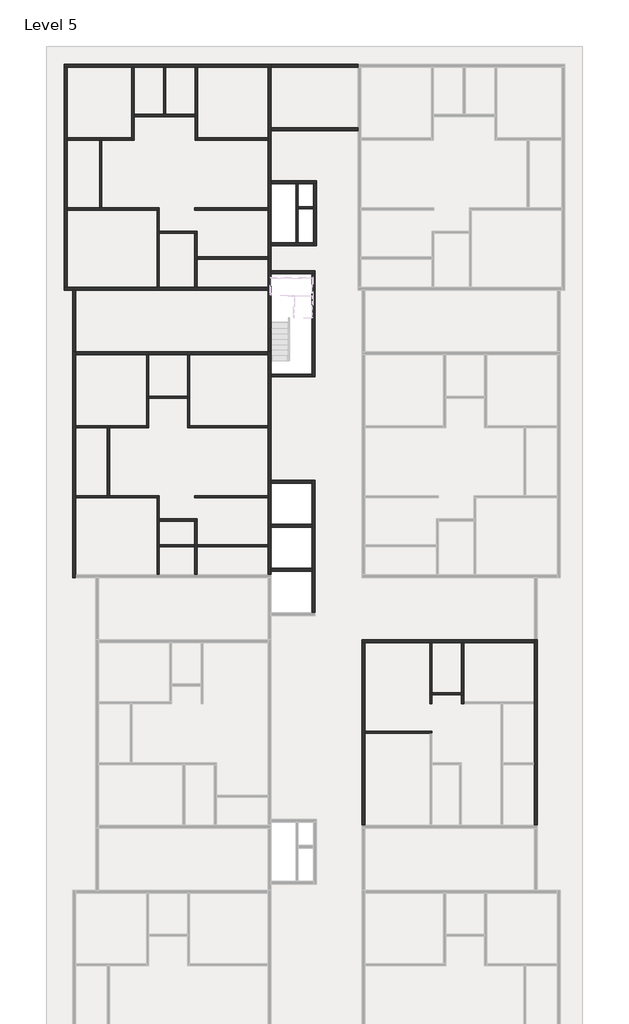
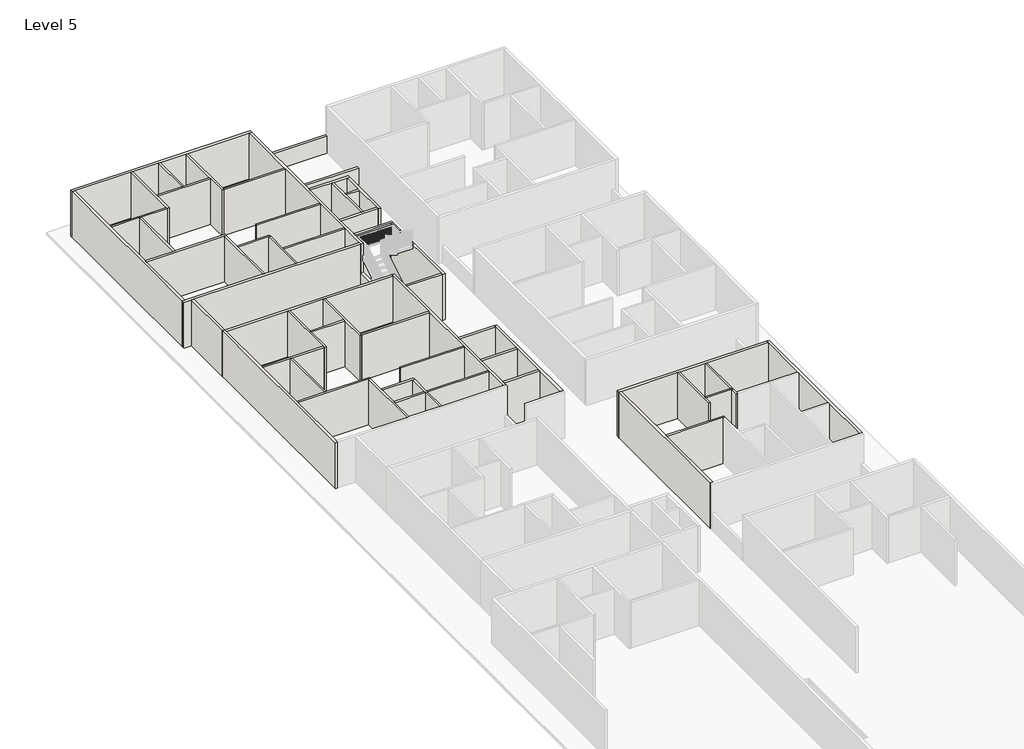
# One storey, part 3 of 8: 57 walls.
"""IFC4 building model written with IfcOpenShell, lengths in millimetres."""

from ifc_helpers import new_model, si_unit, frame, origin, place, context, project, spatial, polyline, outline, extrude, faceted_brep, element, save

model = new_model("IFC4")

# Units and contexts
model_context = context("Model", 3, world=origin())
ifc_project = project(units=[si_unit("LENGTHUNIT", "METRE", prefix="MILLI")], contexts=[model_context])

# Site, building, storey
site = spatial("IfcSite", under=ifc_project)
building = spatial("IfcBuilding", under=site)
storey = spatial("IfcBuildingStorey", under=building, Name="Level 5", Elevation=37426.6172466)

# Walls
placement = place(None, origin())
element("IfcWall", 1, ObjectType="4.5\"", at=placement, inside=storey, context=model_context, shape_type="Brep", body=[
    faceted_brep([(-10818.3415084, 35031.1216096, 37426.6172466), (-10818.3415084, 31373.5216096, 37426.6172466), (-10818.3415084, 31259.2216096, 37426.6172466), (-10818.3415084, 31259.2216096, 40474.6172466), (-10818.3415084, 31373.5216096, 40474.6172466), (-10818.3415084, 35031.1216096, 40474.6172466), (-10704.0415084, 35031.1216096, 37426.6172466), (-10704.0415084, 35031.1216096, 40474.6172466), (-10704.0415084, 32592.7216096, 40474.6172466), (-10704.0415084, 32478.4216096, 40474.6172466), (-10704.0415084, 31259.2216096, 40474.6172466), (-10704.0415084, 31259.2216096, 37426.6172466), (-10704.0415084, 32478.4216096, 37426.6172466), (-10704.0415084, 32592.7216096, 37426.6172466)], [[[0, 1, 2, 3, 4, 5]], [[6, 7, 8, 9, 10, 11, 12, 13]], [[2, 1, 0, 6, 13, 12, 11]], [[0, 5, 7, 6]], [[3, 2, 11, 10]], [[5, 4, 3, 10, 9, 8, 7]]]),
])
element("IfcWall", 2, ObjectType="4.5\"", at=placement, inside=storey, context=model_context, shape_type="Brep", body=[
    faceted_brep([(-10818.3415084, 31373.5216096, 37426.6172466), (-14171.1415084, 31373.5216096, 37426.6172466), (-14171.1415084, 31373.5216096, 40474.6172466), (-10818.3415084, 31373.5216096, 40474.6172466), (-10818.3415084, 31259.2216096, 37426.6172466), (-10818.3415084, 31259.2216096, 40474.6172466), (-12380.4415084, 31259.2216096, 40474.6172466), (-12494.7415084, 31259.2216096, 40474.6172466), (-14171.1415084, 31259.2216096, 40474.6172466), (-14171.1415084, 31259.2216096, 37426.6172466), (-12494.7415084, 31259.2216096, 37426.6172466), (-12380.4415084, 31259.2216096, 37426.6172466)], [[[0, 1, 2, 3]], [[4, 5, 6, 7, 8, 9, 10, 11]], [[1, 0, 4, 11, 10, 9]], [[0, 3, 5, 4]], [[2, 1, 9, 8]], [[3, 2, 8, 7, 6, 5]]]),
])
element("IfcWall", 3, ObjectType="4.5\"", at=placement, inside=storey, context=model_context, shape_type="SweptSolid", body=[
    extrude(outline(polyline([(-12494.7415084, 27754.0216096), (-12494.7415084, 31259.2216096), (-12380.4415084, 31259.2216096), (-12380.4415084, 27754.0216096), (-12494.7415084, 27754.0216096)])), frame((0.0, 0.0, 37426.6172466), z_axis=(0.0, 0.0, 1.0), x_axis=(1.0, 0.0, 0.0)), (0.0, 0.0, 1.0), 3048.0),
])
element("IfcWall", 4, ObjectType="4.5\"", at=placement, inside=storey, context=model_context, shape_type="Brep", body=[
    faceted_brep([(-14171.1415084, 27639.7216096, 37426.6172466), (-9510.2415084, 27639.7216096, 37426.6172466), (-9395.9415084, 27639.7216096, 37426.6172466), (-9395.9415084, 27639.7216096, 40474.6172466), (-9510.2415084, 27639.7216096, 40474.6172466), (-14171.1415084, 27639.7216096, 40474.6172466), (-14171.1415084, 27754.0216096, 37426.6172466), (-14171.1415084, 27754.0216096, 40474.6172466), (-12494.7415084, 27754.0216096, 40474.6172466), (-12380.4415084, 27754.0216096, 40474.6172466), (-9395.9415084, 27754.0216096, 40474.6172466), (-9395.9415084, 27754.0216096, 37426.6172466), (-12380.4415084, 27754.0216096, 37426.6172466), (-12494.7415084, 27754.0216096, 37426.6172466)], [[[0, 1, 2, 3, 4, 5]], [[6, 7, 8, 9, 10, 11, 12, 13]], [[2, 1, 0, 6, 13, 12, 11]], [[0, 5, 7, 6]], [[3, 2, 11, 10]], [[5, 4, 3, 10, 9, 8, 7]]]),
])
element("IfcWall", 5, ObjectType="4.5\"", at=placement, inside=storey, context=model_context, shape_type="Brep", body=[
    faceted_brep([(-9510.2415084, 27639.7216096, 37426.6172466), (-9510.2415084, 23651.9216096, 37426.6172466), (-9510.2415084, 23651.9216096, 40474.6172466), (-9510.2415084, 27639.7216096, 40474.6172466), (-9395.9415084, 27639.7216096, 37426.6172466), (-9395.9415084, 27639.7216096, 40474.6172466), (-9395.9415084, 26547.5216096, 40474.6172466), (-9395.9415084, 26433.2216096, 40474.6172466), (-9395.9415084, 23651.9216096, 40474.6172466), (-9395.9415084, 23651.9216096, 37426.6172466), (-9395.9415084, 26433.2216096, 37426.6172466), (-9395.9415084, 26547.5216096, 37426.6172466)], [[[0, 1, 2, 3]], [[4, 5, 6, 7, 8, 9, 10, 11]], [[1, 0, 4, 11, 10, 9]], [[0, 3, 5, 4]], [[2, 1, 9, 8]], [[3, 2, 8, 7, 6, 5]]]),
])
element("IfcWall", 6, ObjectType="4.5\"", at=placement, inside=storey, context=model_context, shape_type="Brep", body=[
    faceted_brep([(-9395.9415084, 26433.2216096, 37426.6172466), (-7567.1415084, 26433.2216096, 37426.6172466), (-7452.8415084, 26433.2216096, 37426.6172466), (-7452.8415084, 26433.2216096, 40474.6172466), (-7567.1415084, 26433.2216096, 40474.6172466), (-9395.9415084, 26433.2216096, 40474.6172466), (-9395.9415084, 26547.5216096, 37426.6172466), (-9395.9415084, 26547.5216096, 40474.6172466), (-7452.8415084, 26547.5216096, 40474.6172466), (-7452.8415084, 26547.5216096, 37426.6172466)], [[[0, 1, 2, 3, 4, 5]], [[6, 7, 8, 9]], [[2, 1, 0, 6, 9]], [[0, 5, 7, 6]], [[3, 2, 9, 8]], [[5, 4, 3, 8, 7]]]),
])
element("IfcWall", 7, ObjectType="4.5\"", at=placement, inside=storey, context=model_context, shape_type="Brep", body=[
    faceted_brep([(-7567.1415084, 26433.2216096, 37426.6172466), (-7567.1415084, 23651.9216096, 37426.6172466), (-7567.1415084, 23651.9216096, 40474.6172466), (-7567.1415084, 26433.2216096, 40474.6172466), (-7452.8415084, 26433.2216096, 37426.6172466), (-7452.8415084, 26433.2216096, 40474.6172466), (-7452.8415084, 25214.0216096, 40474.6172466), (-7452.8415084, 25099.7216096, 40474.6172466), (-7452.8415084, 23651.9216096, 40474.6172466), (-7452.8415084, 23651.9216096, 37426.6172466), (-7452.8415084, 25099.7216096, 37426.6172466), (-7452.8415084, 25214.0216096, 37426.6172466)], [[[0, 1, 2, 3]], [[4, 5, 6, 7, 8, 9, 10, 11]], [[1, 0, 4, 11, 10, 9]], [[0, 3, 5, 4]], [[2, 1, 9, 8]], [[3, 2, 8, 7, 6, 5]]]),
])
element("IfcWall", 8, ObjectType="4.5\"", at=placement, inside=storey, context=model_context, shape_type="SweptSolid", body=[
    extrude(outline(polyline([(-7452.8415084, 25214.0216096), (-3769.8415084, 25214.0216096), (-3769.8415084, 25099.7216096), (-7452.8415084, 25099.7216096), (-7452.8415084, 25214.0216096)])), frame((0.0, 0.0, 37426.6172466), z_axis=(0.0, 0.0, 1.0), x_axis=(1.0, 0.0, 0.0)), (0.0, 0.0, 1.0), 3048.0),
])
element("IfcWall", 9, ObjectType="4.5\"", at=placement, inside=storey, context=model_context, shape_type="SweptSolid", body=[
    extrude(outline(polyline([(-3769.8415084, 27639.7216096), (-7567.1415084, 27639.7216096), (-7567.1415084, 27754.0216096), (-3769.8415084, 27754.0216096), (-3769.8415084, 27639.7216096)])), frame((0.0, 0.0, 37426.6172466), z_axis=(0.0, 0.0, 1.0), x_axis=(1.0, 0.0, 0.0)), (0.0, 0.0, 1.0), 3048.0),
])
element("IfcWall", 10, ObjectType="4.5\"", at=placement, inside=storey, context=model_context, shape_type="Brep", body=[
    faceted_brep([(-10704.0415084, 32478.4216096, 37426.6172466), (-7541.7415084, 32478.4216096, 37426.6172466), (-7541.7415084, 32478.4216096, 40474.6172466), (-10704.0415084, 32478.4216096, 40474.6172466), (-10704.0415084, 32592.7216096, 37426.6172466), (-10704.0415084, 32592.7216096, 40474.6172466), (-9180.0415084, 32592.7216096, 40474.6172466), (-9065.7415084, 32592.7216096, 40474.6172466), (-7541.7415084, 32592.7216096, 40474.6172466), (-7541.7415084, 32592.7216096, 37426.6172466), (-9065.7415084, 32592.7216096, 37426.6172466), (-9180.0415084, 32592.7216096, 37426.6172466)], [[[0, 1, 2, 3]], [[4, 5, 6, 7, 8, 9, 10, 11]], [[1, 0, 4, 11, 10, 9]], [[0, 3, 5, 4]], [[2, 1, 9, 8]], [[3, 2, 8, 7, 6, 5]]]),
])
element("IfcWall", 11, ObjectType="4.5\"", at=placement, inside=storey, context=model_context, shape_type="SweptSolid", body=[
    extrude(outline(polyline([(-9180.0415084, 32592.7216096), (-9180.0415084, 35031.1216096), (-9065.7415084, 35031.1216096), (-9065.7415084, 32592.7216096), (-9180.0415084, 32592.7216096)])), frame((0.0, 0.0, 37426.6172466), z_axis=(0.0, 0.0, 1.0), x_axis=(1.0, 0.0, 0.0)), (0.0, 0.0, 1.0), 3048.0),
])
element("IfcWall", 12, ObjectType="4.5\"", at=placement, inside=storey, context=model_context, shape_type="Brep", body=[
    faceted_brep([(-7541.7415084, 35031.1216096, 37426.6172466), (-7541.7415084, 32592.7216096, 37426.6172466), (-7541.7415084, 32478.4216096, 37426.6172466), (-7541.7415084, 31259.2216096, 37426.6172466), (-7541.7415084, 31259.2216096, 40474.6172466), (-7541.7415084, 32478.4216096, 40474.6172466), (-7541.7415084, 32592.7216096, 40474.6172466), (-7541.7415084, 35031.1216096, 40474.6172466), (-7427.4415084, 35031.1216096, 37426.6172466), (-7427.4415084, 35031.1216096, 40474.6172466), (-7427.4415084, 31373.5216096, 40474.6172466), (-7427.4415084, 31259.2216096, 40474.6172466), (-7427.4415084, 31259.2216096, 37426.6172466), (-7427.4415084, 31373.5216096, 37426.6172466)], [[[0, 1, 2, 3, 4, 5, 6, 7]], [[8, 9, 10, 11, 12, 13]], [[3, 2, 1, 0, 8, 13, 12]], [[0, 7, 9, 8]], [[4, 3, 12, 11]], [[7, 6, 5, 4, 11, 10, 9]]]),
])
element("IfcWall", 13, ObjectType="4.5\"", at=placement, inside=storey, context=model_context, shape_type="SweptSolid", body=[
    extrude(outline(polyline([(-3769.8415084, 31259.2216096), (-7427.4415084, 31259.2216096), (-7427.4415084, 31373.5216096), (-3769.8415084, 31373.5216096), (-3769.8415084, 31259.2216096)])), frame((0.0, 0.0, 37426.6172466), z_axis=(0.0, 0.0, 1.0), x_axis=(1.0, 0.0, 0.0)), (0.0, 0.0, 1.0), 3048.0),
])
element("IfcWall", 14, ObjectType="4.5\"", at=placement, inside=storey, context=model_context, shape_type="Brep", body=[
    faceted_brep([(-10061.4044854, 20146.7216096, 37426.6172466), (-10061.4044854, 16489.1216096, 37426.6172466), (-10061.4044854, 16374.8216096, 37426.6172466), (-10061.4044854, 16374.8216096, 40474.6172466), (-10061.4044854, 16489.1216096, 40474.6172466), (-10061.4044854, 20146.7216096, 40474.6172466), (-9947.1044854, 20146.7216096, 37426.6172466), (-9947.1044854, 20146.7216096, 40474.6172466), (-9947.1044854, 18013.1216096, 40474.6172466), (-9947.1044854, 17898.8216096, 40474.6172466), (-9947.1044854, 16374.8216096, 40474.6172466), (-9947.1044854, 16374.8216096, 37426.6172466), (-9947.1044854, 17898.8216096, 37426.6172466), (-9947.1044854, 18013.1216096, 37426.6172466)], [[[0, 1, 2, 3, 4, 5]], [[6, 7, 8, 9, 10, 11, 12, 13]], [[2, 1, 0, 6, 13, 12, 11]], [[0, 5, 7, 6]], [[3, 2, 11, 10]], [[5, 4, 3, 10, 9, 8, 7]]]),
])
element("IfcWall", 15, ObjectType="4.5\"", at=placement, inside=storey, context=model_context, shape_type="Brep", body=[
    faceted_brep([(-10061.4044854, 16489.1216096, 37426.6172466), (-13719.0044854, 16489.1216096, 37426.6172466), (-13719.0044854, 16489.1216096, 40474.6172466), (-10061.4044854, 16489.1216096, 40474.6172466), (-10061.4044854, 16374.8216096, 37426.6172466), (-10061.4044854, 16374.8216096, 40474.6172466), (-11980.3915084, 16374.8216096, 40474.6172466), (-12094.6915084, 16374.8216096, 40474.6172466), (-13719.0044854, 16374.8216096, 40474.6172466), (-13719.0044854, 16374.8216096, 37426.6172466), (-12094.6915084, 16374.8216096, 37426.6172466), (-11980.3915084, 16374.8216096, 37426.6172466)], [[[0, 1, 2, 3]], [[4, 5, 6, 7, 8, 9, 10, 11]], [[1, 0, 4, 11, 10, 9]], [[0, 3, 5, 4]], [[2, 1, 9, 8]], [[3, 2, 8, 7, 6, 5]]]),
])
element("IfcWall", 16, ObjectType="4.5\"", at=placement, inside=storey, context=model_context, shape_type="SweptSolid", body=[
    extrude(outline(polyline([(-7940.5044854, 17898.8216096), (-9947.1044854, 17898.8216096), (-9947.1044854, 18013.1216096), (-7940.5044854, 18013.1216096), (-7940.5044854, 17898.8216096)])), frame((0.0, 0.0, 37426.6172466), z_axis=(0.0, 0.0, 1.0), x_axis=(1.0, 0.0, 0.0)), (0.0, 0.0, 1.0), 3048.0),
])
element("IfcWall", 17, ObjectType="4.5\"", at=placement, inside=storey, context=model_context, shape_type="Brep", body=[
    faceted_brep([(-7940.5044854, 20146.7216096, 37426.6172466), (-7940.5044854, 18013.1216096, 37426.6172466), (-7940.5044854, 17898.8216096, 37426.6172466), (-7940.5044854, 16374.8216096, 37426.6172466), (-7940.5044854, 16374.8216096, 40474.6172466), (-7940.5044854, 17898.8216096, 40474.6172466), (-7940.5044854, 18013.1216096, 40474.6172466), (-7940.5044854, 20146.7216096, 40474.6172466), (-7826.2044854, 20146.7216096, 37426.6172466), (-7826.2044854, 20146.7216096, 40474.6172466), (-7826.2044854, 16489.1216096, 40474.6172466), (-7826.2044854, 16374.8216096, 40474.6172466), (-7826.2044854, 16374.8216096, 37426.6172466), (-7826.2044854, 16489.1216096, 37426.6172466)], [[[0, 1, 2, 3, 4, 5, 6, 7]], [[8, 9, 10, 11, 12, 13]], [[3, 2, 1, 0, 8, 13, 12]], [[0, 7, 9, 8]], [[4, 3, 12, 11]], [[7, 6, 5, 4, 11, 10, 9]]]),
])
element("IfcWall", 18, ObjectType="4.5\"", at=placement, inside=storey, context=model_context, shape_type="SweptSolid", body=[
    extrude(outline(polyline([(-3769.8415084, 16374.8216096), (-7826.2044854, 16374.8216096), (-7826.2044854, 16489.1216096), (-3769.8415084, 16489.1216096), (-3769.8415084, 16374.8216096)])), frame((0.0, 0.0, 37426.6172466), z_axis=(0.0, 0.0, 1.0), x_axis=(1.0, 0.0, 0.0)), (0.0, 0.0, 1.0), 3048.0),
])
element("IfcWall", 19, ObjectType="4.5\"", at=placement, inside=storey, context=model_context, shape_type="SweptSolid", body=[
    extrude(outline(polyline([(-12094.6915084, 12869.6216096), (-12094.6915084, 16374.8216096), (-11980.3915084, 16374.8216096), (-11980.3915084, 12869.6216096), (-12094.6915084, 12869.6216096)])), frame((0.0, 0.0, 37426.6172466), z_axis=(0.0, 0.0, 1.0), x_axis=(1.0, 0.0, 0.0)), (0.0, 0.0, 1.0), 3048.0),
])
element("IfcWall", 20, ObjectType="4.5\"", at=placement, inside=storey, context=model_context, shape_type="Brep", body=[
    faceted_brep([(-13719.0044854, 12755.3216096, 37426.6172466), (-9510.2415084, 12755.3216096, 37426.6172466), (-9395.9415084, 12755.3216096, 37426.6172466), (-9395.9415084, 12755.3216096, 40474.6172466), (-9510.2415084, 12755.3216096, 40474.6172466), (-13719.0044854, 12755.3216096, 40474.6172466), (-13719.0044854, 12869.6216096, 37426.6172466), (-13719.0044854, 12869.6216096, 40474.6172466), (-12094.6915084, 12869.6216096, 40474.6172466), (-11980.3915084, 12869.6216096, 40474.6172466), (-9395.9415084, 12869.6216096, 40474.6172466), (-9395.9415084, 12869.6216096, 37426.6172466), (-11980.3915084, 12869.6216096, 37426.6172466), (-12094.6915084, 12869.6216096, 37426.6172466)], [[[0, 1, 2, 3, 4, 5]], [[6, 7, 8, 9, 10, 11, 12, 13]], [[2, 1, 0, 6, 13, 12, 11]], [[0, 5, 7, 6]], [[3, 2, 11, 10]], [[5, 4, 3, 10, 9, 8, 7]]]),
])
element("IfcWall", 21, ObjectType="4.5\"", at=placement, inside=storey, context=model_context, shape_type="Brep", body=[
    faceted_brep([(-9510.2415084, 12755.3216096, 37426.6172466), (-9510.2415084, 8767.5216096, 37426.6172466), (-9510.2415084, 8767.5216096, 40474.6172466), (-9510.2415084, 12755.3216096, 40474.6172466), (-9395.9415084, 12755.3216096, 37426.6172466), (-9395.9415084, 12755.3216096, 40474.6172466), (-9395.9415084, 11663.1216096, 40474.6172466), (-9395.9415084, 11548.8216096, 40474.6172466), (-9395.9415084, 10329.6216096, 40474.6172466), (-9395.9415084, 10215.3216096, 40474.6172466), (-9395.9415084, 8767.5216096, 40474.6172466), (-9395.9415084, 8767.5216096, 37426.6172466), (-9395.9415084, 10215.3216096, 37426.6172466), (-9395.9415084, 10329.6216096, 37426.6172466), (-9395.9415084, 11548.8216096, 37426.6172466), (-9395.9415084, 11663.1216096, 37426.6172466)], [[[0, 1, 2, 3]], [[4, 5, 6, 7, 8, 9, 10, 11, 12, 13, 14, 15]], [[1, 0, 4, 15, 14, 13, 12, 11]], [[0, 3, 5, 4]], [[2, 1, 11, 10]], [[3, 2, 10, 9, 8, 7, 6, 5]]]),
])
element("IfcWall", 22, ObjectType="4.5\"", at=placement, inside=storey, context=model_context, shape_type="SweptSolid", body=[
    extrude(outline(polyline([(-7567.1415084, 10215.3216096), (-9395.9415084, 10215.3216096), (-9395.9415084, 10329.6216096), (-7567.1415084, 10329.6216096), (-7567.1415084, 10215.3216096)])), frame((0.0, 0.0, 37426.6172466), z_axis=(0.0, 0.0, 1.0), x_axis=(1.0, 0.0, 0.0)), (0.0, 0.0, 1.0), 3048.0),
])
element("IfcWall", 23, ObjectType="4.5\"", at=placement, inside=storey, context=model_context, shape_type="Brep", body=[
    faceted_brep([(-9395.9415084, 11548.8216096, 37426.6172466), (-7567.1415084, 11548.8216096, 37426.6172466), (-7452.8415084, 11548.8216096, 37426.6172466), (-7452.8415084, 11548.8216096, 40474.6172466), (-7567.1415084, 11548.8216096, 40474.6172466), (-9395.9415084, 11548.8216096, 40474.6172466), (-9395.9415084, 11663.1216096, 37426.6172466), (-9395.9415084, 11663.1216096, 40474.6172466), (-7452.8415084, 11663.1216096, 40474.6172466), (-7452.8415084, 11663.1216096, 37426.6172466)], [[[0, 1, 2, 3, 4, 5]], [[6, 7, 8, 9]], [[2, 1, 0, 6, 9]], [[0, 5, 7, 6]], [[3, 2, 9, 8]], [[5, 4, 3, 8, 7]]]),
])
element("IfcWall", 24, ObjectType="4.5\"", at=placement, inside=storey, context=model_context, shape_type="Brep", body=[
    faceted_brep([(-7567.1415084, 11548.8216096, 37426.6172466), (-7567.1415084, 10329.6216096, 37426.6172466), (-7567.1415084, 10215.3216096, 37426.6172466), (-7567.1415084, 8767.5216096, 37426.6172466), (-7567.1415084, 8767.5216096, 40474.6172466), (-7567.1415084, 10215.3216096, 40474.6172466), (-7567.1415084, 10329.6216096, 40474.6172466), (-7567.1415084, 11548.8216096, 40474.6172466), (-7452.8415084, 11548.8216096, 37426.6172466), (-7452.8415084, 11548.8216096, 40474.6172466), (-7452.8415084, 10329.6216096, 40474.6172466), (-7452.8415084, 10215.3216096, 40474.6172466), (-7452.8415084, 8767.5216096, 40474.6172466), (-7452.8415084, 8767.5216096, 37426.6172466), (-7452.8415084, 10215.3216096, 37426.6172466), (-7452.8415084, 10329.6216096, 37426.6172466)], [[[0, 1, 2, 3, 4, 5, 6, 7]], [[8, 9, 10, 11, 12, 13, 14, 15]], [[3, 2, 1, 0, 8, 15, 14, 13]], [[0, 7, 9, 8]], [[4, 3, 13, 12]], [[7, 6, 5, 4, 12, 11, 10, 9]]]),
])
element("IfcWall", 25, ObjectType="4.5\"", at=placement, inside=storey, context=model_context, shape_type="SweptSolid", body=[
    extrude(outline(polyline([(-3769.8415084, 10215.3216096), (-7452.8415084, 10215.3216096), (-7452.8415084, 10329.6216096), (-3769.8415084, 10329.6216096), (-3769.8415084, 10215.3216096)])), frame((0.0, 0.0, 37426.6172466), z_axis=(0.0, 0.0, 1.0), x_axis=(1.0, 0.0, 0.0)), (0.0, 0.0, 1.0), 3048.0),
])
element("IfcWall", 26, ObjectType="4.5\"", at=placement, inside=storey, context=model_context, shape_type="SweptSolid", body=[
    extrude(outline(polyline([(-3769.8415084, 12755.3216096), (-7567.1415084, 12755.3216096), (-7567.1415084, 12869.6216096), (-3769.8415084, 12869.6216096), (-3769.8415084, 12755.3216096)])), frame((0.0, 0.0, 37426.6172466), z_axis=(0.0, 0.0, 1.0), x_axis=(1.0, 0.0, 0.0)), (0.0, 0.0, 1.0), 3048.0),
])
element("IfcWall", 27, ObjectType="4.5\"", at=placement, inside=storey, context=model_context, shape_type="Brep", body=[
    faceted_brep([(1259.3584916, 572.7745083, 37426.6172466), (4610.8714687, 572.7745083, 37426.6172466), (4725.1714687, 572.7745083, 37426.6172466), (4725.1714687, 572.7745083, 40474.6172466), (4610.8714687, 572.7745083, 40474.6172466), (1259.3584916, 572.7745083, 40474.6172466), (1259.3584916, 687.0745083, 37426.6172466), (1259.3584916, 687.0745083, 40474.6172466), (4725.1714687, 687.0745083, 40474.6172466), (4725.1714687, 687.0745083, 37426.6172466)], [[[0, 1, 2, 3, 4, 5]], [[6, 7, 8, 9]], [[2, 1, 0, 6, 9]], [[0, 5, 7, 6]], [[3, 2, 9, 8]], [[5, 4, 3, 8, 7]]]),
])
element("IfcWall", 28, ObjectType="4.5\"", at=placement, inside=storey, context=model_context, shape_type="Brep", body=[
    faceted_brep([(4610.8714687, 5262.3216096, 37426.6172466), (4610.8714687, 2100.0216096, 37426.6172466), (4610.8714687, 2100.0216096, 40474.6172466), (4610.8714687, 5262.3216096, 40474.6172466), (4725.1714687, 5262.3216096, 37426.6172466), (4725.1714687, 5262.3216096, 40474.6172466), (4725.1714687, 2671.5216096, 40474.6172466), (4725.1714687, 2557.2216096, 40474.6172466), (4725.1714687, 2100.0216096, 40474.6172466), (4725.1714687, 2100.0216096, 37426.6172466), (4725.1714687, 2557.2216096, 37426.6172466), (4725.1714687, 2671.5216096, 37426.6172466)], [[[0, 1, 2, 3]], [[4, 5, 6, 7, 8, 9, 10, 11]], [[1, 0, 4, 11, 10, 9]], [[2, 1, 9, 8]], [[0, 3, 5, 4]], [[3, 2, 8, 7, 6, 5]]]),
])
element("IfcWall", 29, ObjectType="4.5\"", at=placement, inside=storey, context=model_context, shape_type="Brep", body=[
    faceted_brep([(4725.1714687, 2557.2216096, 37426.6172466), (6249.1714687, 2557.2216096, 37426.6172466), (6363.4714687, 2557.2216096, 37426.6172466), (6363.4714687, 2557.2216096, 40474.6172466), (6249.1714687, 2557.2216096, 40474.6172466), (4725.1714687, 2557.2216096, 40474.6172466), (4725.1714687, 2671.5216096, 37426.6172466), (4725.1714687, 2671.5216096, 40474.6172466), (6249.1714687, 2671.5216096, 40474.6172466), (6363.4714687, 2671.5216096, 40474.6172466), (6363.4714687, 2671.5216096, 37426.6172466), (6249.1714687, 2671.5216096, 37426.6172466)], [[[0, 1, 2, 3, 4, 5]], [[6, 7, 8, 9, 10, 11]], [[2, 1, 0, 6, 11, 10]], [[0, 5, 7, 6]], [[3, 2, 10, 9]], [[5, 4, 3, 9, 8, 7]]]),
])
element("IfcWall", 30, ObjectType="4.5\"", at=placement, inside=storey, context=model_context, shape_type="SweptSolid", body=[
    extrude(outline(polyline([(6363.4714687, 5262.3216096), (6363.4714687, 2671.5216096), (6249.1714687, 2671.5216096), (6249.1714687, 5262.3216096), (6363.4714687, 5262.3216096)])), frame((0.0, 0.0, 37426.6172466), z_axis=(0.0, 0.0, 1.0), x_axis=(1.0, 0.0, 0.0)), (0.0, 0.0, 1.0), 3048.0),
])
element("IfcWall", 31, ObjectType="4.5\"", at=placement, inside=storey, context=model_context, shape_type="Brep", body=[
    faceted_brep([(6249.1714687, 2557.2216096, 37426.6172466), (6249.1714687, 2100.0216096, 37426.6172466), (6249.1714687, 2100.0216096, 40474.6172466), (6249.1714687, 2557.2216096, 40474.6172466), (6363.4714687, 2557.2216096, 37426.6172466), (6363.4714687, 2557.2216096, 40474.6172466), (6363.4714687, 2214.3216096, 40474.6172466), (6363.4714687, 2100.0216096, 40474.6172466), (6363.4714687, 2100.0216096, 37426.6172466), (6363.4714687, 2214.3216096, 37426.6172466)], [[[0, 1, 2, 3]], [[4, 5, 6, 7, 8, 9]], [[1, 0, 4, 9, 8]], [[0, 3, 5, 4]], [[2, 1, 8, 7]], [[3, 2, 7, 6, 5]]]),
])
element("IfcWall", 32, ObjectType="4.5\"", at=placement, inside=storey, context=model_context, shape_type="Brep", body=[
    faceted_brep([(-2321.9738684, 29000.0900967, 37426.6172466), (-2321.9738684, 25952.0900967, 37426.6172466), (-2321.9738684, 25952.0900967, 40474.6172466), (-2321.9738684, 29000.0900967, 40474.6172466), (-2207.6738684, 29000.0900967, 37426.6172466), (-2207.6738684, 29000.0900967, 40474.6172466), (-2207.6738684, 27820.8172885, 40474.6172466), (-2207.6738684, 27706.5172885, 40474.6172466), (-2207.6738684, 25952.0900967, 40474.6172466), (-2207.6738684, 25952.0900967, 37426.6172466), (-2207.6738684, 27706.5172885, 37426.6172466), (-2207.6738684, 27820.8172885, 37426.6172466)], [[[0, 1, 2, 3]], [[4, 5, 6, 7, 8, 9, 10, 11]], [[1, 0, 4, 11, 10, 9]], [[3, 2, 8, 7, 6, 5]], [[0, 3, 5, 4]], [[2, 1, 9, 8]]]),
])
element("IfcWall", 33, ObjectType="4.5\"", at=placement, inside=storey, context=model_context, shape_type="SweptSolid", body=[
    extrude(outline(polyline([(-2207.6738684, 27820.8172885), (-1407.6415084, 27820.8172885), (-1407.6415084, 27706.5172885), (-2207.6738684, 27706.5172885), (-2207.6738684, 27820.8172885)])), frame((0.0, 0.0, 37426.6172466), z_axis=(0.0, 0.0, 1.0), x_axis=(1.0, 0.0, 0.0)), (0.0, 0.0, 1.0), 3048.0),
])
element("IfcWall", 34, ObjectType="6\"", at=placement, inside=storey, context=model_context, shape_type="Brep", body=[
    faceted_brep([(-14323.5415084, 35031.1216096, 37426.6172466), (-14171.1415084, 35031.1216096, 37426.6172466), (-10818.3415084, 35031.1216096, 37426.6172466), (-10704.0415084, 35031.1216096, 37426.6172466), (-9180.0415084, 35031.1216096, 37426.6172466), (-9065.7415084, 35031.1216096, 37426.6172466), (-7541.7415084, 35031.1216096, 37426.6172466), (-7427.4415084, 35031.1216096, 37426.6172466), (-3769.8415084, 35031.1216096, 37426.6172466), (-3617.4415084, 35031.1216096, 37426.6172466), (-3617.4415084, 35031.1216096, 40474.6172466), (-3769.8415084, 35031.1216096, 40474.6172466), (-7427.4415084, 35031.1216096, 40474.6172466), (-7541.7415084, 35031.1216096, 40474.6172466), (-9065.7415084, 35031.1216096, 40474.6172466), (-9180.0415084, 35031.1216096, 40474.6172466), (-10704.0415084, 35031.1216096, 40474.6172466), (-10818.3415084, 35031.1216096, 40474.6172466), (-14171.1415084, 35031.1216096, 40474.6172466), (-14323.5415084, 35031.1216096, 40474.6172466), (-14323.5415084, 35183.5216096, 37426.6172466), (-14323.5415084, 35183.5216096, 40474.6172466), (-3617.4415084, 35183.5216096, 40474.6172466), (-3617.4415084, 35183.5216096, 37426.6172466)], [[[0, 1, 2, 3, 4, 5, 6, 7, 8, 9, 10, 11, 12, 13, 14, 15, 16, 17, 18, 19]], [[20, 21, 22, 23]], [[9, 8, 7, 6, 5, 4, 3, 2, 1, 0, 20, 23]], [[0, 19, 21, 20]], [[9, 23, 22, 10]], [[19, 18, 17, 16, 15, 14, 13, 12, 11, 10, 22, 21]]]),
])
element("IfcWall", 35, ObjectType="6\"", at=placement, inside=storey, context=model_context, shape_type="Brep", body=[
    faceted_brep([(-3769.8415084, 35031.1216096, 40474.6172466), (-3769.8415084, 35031.1216096, 37426.6172466), (-3769.8415084, 31373.5216096, 37426.6172466), (-3769.8415084, 31259.2216096, 37426.6172466), (-3769.8415084, 27754.0216096, 37426.6172466), (-3769.8415084, 27639.7216096, 37426.6172466), (-3769.8415084, 25214.0216096, 37426.6172466), (-3769.8415084, 25099.7216096, 37426.6172466), (-3769.8415084, 23651.9216096, 37426.6172466), (-3769.8415084, 23499.5216096, 37426.6172466), (-3769.8415084, 23499.5216096, 40474.6172466), (-3769.8415084, 23651.9216096, 40474.6172466), (-3769.8415084, 25099.7216096, 40474.6172466), (-3769.8415084, 25214.0216096, 40474.6172466), (-3769.8415084, 27639.7216096, 40474.6172466), (-3769.8415084, 27754.0216096, 40474.6172466), (-3769.8415084, 31259.2216096, 40474.6172466), (-3769.8415084, 31373.5216096, 40474.6172466), (-3617.4415084, 35031.1216096, 37426.6172466), (-3617.4415084, 35031.1216096, 40474.6172466), (-3617.4415084, 29152.4900967, 40474.6172466), (-3617.4415084, 29000.0900967, 40474.6172466), (-3617.4415084, 25952.0900967, 40474.6172466), (-3617.4415084, 25799.6900967, 40474.6172466), (-3617.4415084, 24490.1216096, 40474.6172466), (-3617.4415084, 24337.7216096, 40474.6172466), (-3617.4415084, 23499.5216096, 40474.6172466), (-3617.4415084, 23499.5216096, 37426.6172466), (-3617.4415084, 24337.7216096, 37426.6172466), (-3617.4415084, 24490.1216096, 37426.6172466), (-3617.4415084, 25799.6900967, 37426.6172466), (-3617.4415084, 25952.0900967, 37426.6172466), (-3617.4415084, 29000.0900967, 37426.6172466), (-3617.4415084, 29152.4900967, 37426.6172466), (-3617.4415084, 31744.9197155, 37426.6172466), (-3617.4415084, 31897.3197155, 37426.6172466)], [[[0, 1, 2, 3, 4, 5, 6, 7, 8, 9, 10, 11, 12, 13, 14, 15, 16, 17]], [[18, 19, 20, 21, 22, 23, 24, 25, 26, 27, 28, 29, 30, 31, 32, 33, 34, 35]], [[9, 8, 7, 6, 5, 4, 3, 2, 1, 18, 35, 34, 33, 32, 31, 30, 29, 28, 27]], [[0, 19, 18, 1]], [[9, 27, 26, 10]], [[0, 17, 16, 15, 14, 13, 12, 11, 10, 26, 25, 24, 23, 22, 21, 20, 19]]]),
])
element("IfcWall", 36, ObjectType="6\"", at=placement, inside=storey, context=model_context, shape_type="Brep", body=[
    faceted_brep([(-3769.8415084, 23651.9216096, 40474.6172466), (-3769.8415084, 23651.9216096, 37426.6172466), (-7452.8415084, 23651.9216096, 37426.6172466), (-7567.1415084, 23651.9216096, 37426.6172466), (-9395.9415084, 23651.9216096, 37426.6172466), (-9510.2415084, 23651.9216096, 37426.6172466), (-14171.1415084, 23651.9216096, 37426.6172466), (-14323.5415084, 23651.9216096, 37426.6172466), (-14323.5415084, 23651.9216096, 40474.6172466), (-14171.1415084, 23651.9216096, 40474.6172466), (-9510.2415084, 23651.9216096, 40474.6172466), (-9395.9415084, 23651.9216096, 40474.6172466), (-7567.1415084, 23651.9216096, 40474.6172466), (-7452.8415084, 23651.9216096, 40474.6172466), (-3769.8415084, 23499.5216096, 37426.6172466), (-3769.8415084, 23499.5216096, 40474.6172466), (-13719.0044854, 23499.5216096, 40474.6172466), (-13871.4044854, 23499.5216096, 40474.6172466), (-14323.5415084, 23499.5216096, 40474.6172466), (-14323.5415084, 23499.5216096, 37426.6172466), (-13871.4044854, 23499.5216096, 37426.6172466), (-13719.0044854, 23499.5216096, 37426.6172466)], [[[0, 1, 2, 3, 4, 5, 6, 7, 8, 9, 10, 11, 12, 13]], [[14, 15, 16, 17, 18, 19, 20, 21]], [[7, 6, 5, 4, 3, 2, 1, 14, 21, 20, 19]], [[8, 7, 19, 18]], [[0, 15, 14, 1]], [[0, 13, 12, 11, 10, 9, 8, 18, 17, 16, 15]]]),
])
element("IfcWall", 37, ObjectType="6\"", at=placement, inside=storey, context=model_context, shape_type="Brep", body=[
    faceted_brep([(-14171.1415084, 23651.9216096, 37426.6172466), (-14171.1415084, 27639.7216096, 37426.6172466), (-14171.1415084, 27754.0216096, 37426.6172466), (-14171.1415084, 31259.2216096, 37426.6172466), (-14171.1415084, 31373.5216096, 37426.6172466), (-14171.1415084, 35031.1216096, 37426.6172466), (-14171.1415084, 35031.1216096, 40474.6172466), (-14171.1415084, 31373.5216096, 40474.6172466), (-14171.1415084, 31259.2216096, 40474.6172466), (-14171.1415084, 27754.0216096, 40474.6172466), (-14171.1415084, 27639.7216096, 40474.6172466), (-14171.1415084, 23651.9216096, 40474.6172466), (-14323.5415084, 23651.9216096, 37426.6172466), (-14323.5415084, 23651.9216096, 40474.6172466), (-14323.5415084, 35031.1216096, 40474.6172466), (-14323.5415084, 35031.1216096, 37426.6172466)], [[[0, 1, 2, 3, 4, 5, 6, 7, 8, 9, 10, 11]], [[12, 13, 14, 15]], [[5, 4, 3, 2, 1, 0, 12, 15]], [[6, 5, 15, 14]], [[0, 11, 13, 12]], [[11, 10, 9, 8, 7, 6, 14, 13]]]),
])
element("IfcWall", 38, ObjectType="6\"", at=placement, inside=storey, context=model_context, shape_type="Brep", body=[
    faceted_brep([(-13871.4044854, 20299.1216096, 37426.6172466), (-13871.4044854, 8615.1216096, 37426.6172466), (-13871.4044854, 8615.1216096, 40474.6172466), (-13871.4044854, 20299.1216096, 40474.6172466), (-13719.0044854, 20299.1216096, 37426.6172466), (-13719.0044854, 20299.1216096, 40474.6172466), (-13719.0044854, 20146.7216096, 40474.6172466), (-13719.0044854, 16489.1216096, 40474.6172466), (-13719.0044854, 16374.8216096, 40474.6172466), (-13719.0044854, 12869.6216096, 40474.6172466), (-13719.0044854, 12755.3216096, 40474.6172466), (-13719.0044854, 8767.5216096, 40474.6172466), (-13719.0044854, 8615.1216096, 40474.6172466), (-13719.0044854, 8615.1216096, 37426.6172466), (-13719.0044854, 8767.5216096, 37426.6172466), (-13719.0044854, 12755.3216096, 37426.6172466), (-13719.0044854, 12869.6216096, 37426.6172466), (-13719.0044854, 16374.8216096, 37426.6172466), (-13719.0044854, 16489.1216096, 37426.6172466), (-13719.0044854, 20146.7216096, 37426.6172466)], [[[0, 1, 2, 3]], [[4, 5, 6, 7, 8, 9, 10, 11, 12, 13, 14, 15, 16, 17, 18, 19]], [[1, 0, 4, 19, 18, 17, 16, 15, 14, 13]], [[2, 1, 13, 12]], [[0, 3, 5, 4]], [[3, 2, 12, 11, 10, 9, 8, 7, 6, 5]]]),
])
element("IfcWall", 39, ObjectType="6\"", at=placement, inside=storey, context=model_context, shape_type="Brep", body=[
    faceted_brep([(-3617.4415084, 8767.5216096, 40474.6172466), (-3617.4415084, 8767.5216096, 37426.6172466), (-3617.4415084, 8945.2303368, 37426.6172466), (-3617.4415084, 9097.6303368, 37426.6172466), (-3617.4415084, 11231.2303368, 37426.6172466), (-3617.4415084, 11383.6303368, 37426.6172466), (-3617.4415084, 13517.2303368, 37426.6172466), (-3617.4415084, 13669.6303368, 37426.6172466), (-3617.4415084, 19003.7216096, 37426.6172466), (-3617.4415084, 19156.1216096, 37426.6172466), (-3617.4415084, 20299.1216096, 37426.6172466), (-3617.4415084, 20299.1216096, 40474.6172466), (-3617.4415084, 19156.1216096, 40474.6172466), (-3617.4415084, 19003.7216096, 40474.6172466), (-3617.4415084, 13669.6303368, 40474.6172466), (-3617.4415084, 13517.2303368, 40474.6172466), (-3617.4415084, 11383.6303368, 40474.6172466), (-3617.4415084, 11231.2303368, 40474.6172466), (-3617.4415084, 9097.6303368, 40474.6172466), (-3617.4415084, 8945.2303368, 40474.6172466), (-3769.8415084, 8767.5216096, 37426.6172466), (-3769.8415084, 8767.5216096, 40474.6172466), (-3769.8415084, 10215.3216096, 40474.6172466), (-3769.8415084, 10329.6216096, 40474.6172466), (-3769.8415084, 12755.3216096, 40474.6172466), (-3769.8415084, 12869.6216096, 40474.6172466), (-3769.8415084, 16374.8216096, 40474.6172466), (-3769.8415084, 16489.1216096, 40474.6172466), (-3769.8415084, 20146.7216096, 40474.6172466), (-3769.8415084, 20299.1216096, 40474.6172466), (-3769.8415084, 20299.1216096, 37426.6172466), (-3769.8415084, 20146.7216096, 37426.6172466), (-3769.8415084, 16489.1216096, 37426.6172466), (-3769.8415084, 16374.8216096, 37426.6172466), (-3769.8415084, 12869.6216096, 37426.6172466), (-3769.8415084, 12755.3216096, 37426.6172466), (-3769.8415084, 10329.6216096, 37426.6172466), (-3769.8415084, 10215.3216096, 37426.6172466)], [[[0, 1, 2, 3, 4, 5, 6, 7, 8, 9, 10, 11, 12, 13, 14, 15, 16, 17, 18, 19]], [[20, 21, 22, 23, 24, 25, 26, 27, 28, 29, 30, 31, 32, 33, 34, 35, 36, 37]], [[10, 9, 8, 7, 6, 5, 4, 3, 2, 1, 20, 37, 36, 35, 34, 33, 32, 31, 30]], [[10, 30, 29, 11]], [[0, 21, 20, 1]], [[0, 19, 18, 17, 16, 15, 14, 13, 12, 11, 29, 28, 27, 26, 25, 24, 23, 22, 21]]]),
])
element("IfcWall", 40, ObjectType="6\"", at=placement, inside=storey, context=model_context, shape_type="Brep", body=[
    faceted_brep([(-3769.8415084, 20299.1216096, 40474.6172466), (-3769.8415084, 20299.1216096, 37426.6172466), (-13719.0044854, 20299.1216096, 37426.6172466), (-13719.0044854, 20299.1216096, 40474.6172466), (-3769.8415084, 20146.7216096, 37426.6172466), (-3769.8415084, 20146.7216096, 40474.6172466), (-7826.2044854, 20146.7216096, 40474.6172466), (-7940.5044854, 20146.7216096, 40474.6172466), (-9947.1044854, 20146.7216096, 40474.6172466), (-10061.4044854, 20146.7216096, 40474.6172466), (-13719.0044854, 20146.7216096, 40474.6172466), (-13719.0044854, 20146.7216096, 37426.6172466), (-10061.4044854, 20146.7216096, 37426.6172466), (-9947.1044854, 20146.7216096, 37426.6172466), (-7940.5044854, 20146.7216096, 37426.6172466), (-7826.2044854, 20146.7216096, 37426.6172466)], [[[0, 1, 2, 3]], [[4, 5, 6, 7, 8, 9, 10, 11, 12, 13, 14, 15]], [[2, 1, 4, 15, 14, 13, 12, 11]], [[3, 2, 11, 10]], [[0, 5, 4, 1]], [[0, 3, 10, 9, 8, 7, 6, 5]]]),
])
element("IfcWall", 41, ObjectType="6\"", at=placement, inside=storey, context=model_context, shape_type="Brep", body=[
    faceted_brep([(10173.4714687, -4185.9344126, 40474.6172466), (10173.4714687, -4185.9344126, 37426.6172466), (10173.4714687, 5414.7216096, 37426.6172466), (10173.4714687, 5414.7216096, 40474.6172466), (10021.0714687, -4185.9344126, 37426.6172466), (10021.0714687, -4185.9344126, 40474.6172466), (10021.0714687, -1061.7344126, 40474.6172466), (10021.0714687, -947.4344126, 40474.6172466), (10021.0714687, 2100.0216096, 40474.6172466), (10021.0714687, 2214.3216096, 40474.6172466), (10021.0714687, 5262.3216096, 40474.6172466), (10021.0714687, 5414.7216096, 40474.6172466), (10021.0714687, 5414.7216096, 37426.6172466), (10021.0714687, 5262.3216096, 37426.6172466), (10021.0714687, 2214.3216096, 37426.6172466), (10021.0714687, 2100.0216096, 37426.6172466), (10021.0714687, -947.4344126, 37426.6172466), (10021.0714687, -1061.7344126, 37426.6172466)], [[[0, 1, 2, 3]], [[4, 5, 6, 7, 8, 9, 10, 11, 12, 13, 14, 15, 16, 17]], [[2, 1, 4, 17, 16, 15, 14, 13, 12]], [[2, 12, 11, 3]], [[0, 5, 4, 1]], [[0, 3, 11, 10, 9, 8, 7, 6, 5]]]),
])
element("IfcWall", 42, ObjectType="6\"", at=placement, inside=storey, context=model_context, shape_type="Brep", body=[
    faceted_brep([(10021.0714687, 5414.7216096, 40474.6172466), (10021.0714687, 5414.7216096, 37426.6172466), (1106.9584916, 5414.7216096, 37426.6172466), (1106.9584916, 5414.7216096, 40474.6172466), (10021.0714687, 5262.3216096, 37426.6172466), (10021.0714687, 5262.3216096, 40474.6172466), (6363.4714687, 5262.3216096, 40474.6172466), (6249.1714687, 5262.3216096, 40474.6172466), (4725.1714687, 5262.3216096, 40474.6172466), (4610.8714687, 5262.3216096, 40474.6172466), (1259.3584916, 5262.3216096, 40474.6172466), (1106.9584916, 5262.3216096, 40474.6172466), (1106.9584916, 5262.3216096, 37426.6172466), (1259.3584916, 5262.3216096, 37426.6172466), (4610.8714687, 5262.3216096, 37426.6172466), (4725.1714687, 5262.3216096, 37426.6172466), (6249.1714687, 5262.3216096, 37426.6172466), (6363.4714687, 5262.3216096, 37426.6172466)], [[[0, 1, 2, 3]], [[4, 5, 6, 7, 8, 9, 10, 11, 12, 13, 14, 15, 16, 17]], [[2, 1, 4, 17, 16, 15, 14, 13, 12]], [[3, 2, 12, 11]], [[0, 5, 4, 1]], [[0, 3, 11, 10, 9, 8, 7, 6, 5]]]),
])
element("IfcWall", 43, ObjectType="6\"", at=placement, inside=storey, context=model_context, shape_type="Brep", body=[
    faceted_brep([(1106.9584916, 5262.3216096, 37426.6172466), (1106.9584916, -4185.9344126, 37426.6172466), (1106.9584916, -4185.9344126, 40474.6172466), (1106.9584916, 5262.3216096, 40474.6172466), (1259.3584916, 5262.3216096, 37426.6172466), (1259.3584916, 5262.3216096, 40474.6172466), (1259.3584916, 687.0745083, 40474.6172466), (1259.3584916, 572.7745083, 40474.6172466), (1259.3584916, -4185.9344126, 40474.6172466), (1259.3584916, -4185.9344126, 37426.6172466), (1259.3584916, 572.7745083, 37426.6172466), (1259.3584916, 687.0745083, 37426.6172466)], [[[0, 1, 2, 3]], [[4, 5, 6, 7, 8, 9, 10, 11]], [[1, 0, 4, 11, 10, 9]], [[0, 3, 5, 4]], [[1, 9, 8, 2]], [[3, 2, 8, 7, 6, 5]]]),
])
element("IfcWall", 44, ObjectType="6\"", at=placement, inside=storey, context=model_context, shape_type="Brep", body=[
    faceted_brep([(-1331.4415084, 6811.6303368, 37426.6172466), (-1331.4415084, 13669.6303368, 37426.6172466), (-1331.4415084, 13669.6303368, 40474.6172466), (-1331.4415084, 6811.6303368, 40474.6172466), (-1483.8415084, 6811.6303368, 37426.6172466), (-1483.8415084, 6811.6303368, 40474.6172466), (-1483.8415084, 8945.2303368, 40474.6172466), (-1483.8415084, 9097.6303368, 40474.6172466), (-1483.8415084, 11231.2303368, 40474.6172466), (-1483.8415084, 11383.6303368, 40474.6172466), (-1483.8415084, 13517.2303368, 40474.6172466), (-1483.8415084, 13669.6303368, 40474.6172466), (-1483.8415084, 13669.6303368, 37426.6172466), (-1483.8415084, 13517.2303368, 37426.6172466), (-1483.8415084, 11383.6303368, 37426.6172466), (-1483.8415084, 11231.2303368, 37426.6172466), (-1483.8415084, 9097.6303368, 37426.6172466), (-1483.8415084, 8945.2303368, 37426.6172466)], [[[0, 1, 2, 3]], [[4, 5, 6, 7, 8, 9, 10, 11, 12, 13, 14, 15, 16, 17]], [[1, 0, 4, 17, 16, 15, 14, 13, 12]], [[3, 2, 11, 10, 9, 8, 7, 6, 5]], [[0, 3, 5, 4]], [[2, 1, 12, 11]]]),
])
element("IfcWall", 45, ObjectType="6\"", at=placement, inside=storey, context=model_context, shape_type="SweptSolid", body=[
    extrude(outline(polyline([(-3617.4415084, 13669.6303368), (-1483.8415084, 13669.6303368), (-1483.8415084, 13517.2303368), (-3617.4415084, 13517.2303368), (-3617.4415084, 13669.6303368)])), frame((0.0, 0.0, 37426.6172466), z_axis=(0.0, 0.0, 1.0), x_axis=(1.0, 0.0, 0.0)), (0.0, 0.0, 1.0), 3048.0),
])
element("IfcWall", 46, ObjectType="6\"", at=placement, inside=storey, context=model_context, shape_type="SweptSolid", body=[
    extrude(outline(polyline([(-1483.8415084, 8945.2303368), (-3617.4415084, 8945.2303368), (-3617.4415084, 9097.6303368), (-1483.8415084, 9097.6303368), (-1483.8415084, 8945.2303368)])), frame((0.0, 0.0, 37426.6172466), z_axis=(0.0, 0.0, 1.0), x_axis=(1.0, 0.0, 0.0)), (0.0, 0.0, 1.0), 3048.0),
])
element("IfcWall", 47, ObjectType="6\"", at=placement, inside=storey, context=model_context, shape_type="SweptSolid", body=[
    extrude(outline(polyline([(-3617.4415084, 11383.6303368), (-1483.8415084, 11383.6303368), (-1483.8415084, 11231.2303368), (-3617.4415084, 11231.2303368), (-3617.4415084, 11383.6303368)])), frame((0.0, 0.0, 37426.6172466), z_axis=(0.0, 0.0, 1.0), x_axis=(1.0, 0.0, 0.0)), (0.0, 0.0, 1.0), 3048.0),
])
element("IfcWall", 48, ObjectType="6\"", at=placement, inside=storey, context=model_context, shape_type="Brep", body=[
    faceted_brep([(-3617.4415084, 29000.0900967, 37426.6172466), (-2321.9738684, 29000.0900967, 37426.6172466), (-2207.6738684, 29000.0900967, 37426.6172466), (-1407.6415084, 29000.0900967, 37426.6172466), (-1255.2415084, 29000.0900967, 37426.6172466), (-1255.2415084, 29000.0900967, 40474.6172466), (-1407.6415084, 29000.0900967, 40474.6172466), (-2207.6738684, 29000.0900967, 40474.6172466), (-2321.9738684, 29000.0900967, 40474.6172466), (-3617.4415084, 29000.0900967, 40474.6172466), (-3617.4415084, 29152.4900967, 37426.6172466), (-3617.4415084, 29152.4900967, 40474.6172466), (-1255.2415084, 29152.4900967, 40474.6172466), (-1255.2415084, 29152.4900967, 37426.6172466)], [[[0, 1, 2, 3, 4, 5, 6, 7, 8, 9]], [[10, 11, 12, 13]], [[4, 3, 2, 1, 0, 10, 13]], [[9, 8, 7, 6, 5, 12, 11]], [[0, 9, 11, 10]], [[5, 4, 13, 12]]]),
])
element("IfcWall", 49, ObjectType="6\"", at=placement, inside=storey, context=model_context, shape_type="Brep", body=[
    faceted_brep([(-1407.6415084, 29000.0900967, 37426.6172466), (-1407.6415084, 27820.8172885, 37426.6172466), (-1407.6415084, 27706.5172885, 37426.6172466), (-1407.6415084, 25952.0900967, 37426.6172466), (-1407.6415084, 25799.6900967, 37426.6172466), (-1407.6415084, 25799.6900967, 40474.6172466), (-1407.6415084, 25952.0900967, 40474.6172466), (-1407.6415084, 27706.5172885, 40474.6172466), (-1407.6415084, 27820.8172885, 40474.6172466), (-1407.6415084, 29000.0900967, 40474.6172466), (-1255.2415084, 29000.0900967, 37426.6172466), (-1255.2415084, 29000.0900967, 40474.6172466), (-1255.2415084, 25799.6900967, 40474.6172466), (-1255.2415084, 25799.6900967, 37426.6172466)], [[[0, 1, 2, 3, 4, 5, 6, 7, 8, 9]], [[10, 11, 12, 13]], [[4, 3, 2, 1, 0, 10, 13]], [[9, 8, 7, 6, 5, 12, 11]], [[0, 9, 11, 10]], [[5, 4, 13, 12]]]),
])
element("IfcWall", 50, ObjectType="6\"", at=placement, inside=storey, context=model_context, shape_type="Brep", body=[
    faceted_brep([(-1407.6415084, 25952.0900967, 37426.6172466), (-2207.6738684, 25952.0900967, 37426.6172466), (-2321.9738684, 25952.0900967, 37426.6172466), (-3617.4415084, 25952.0900967, 37426.6172466), (-3617.4415084, 25952.0900967, 40474.6172466), (-2321.9738684, 25952.0900967, 40474.6172466), (-2207.6738684, 25952.0900967, 40474.6172466), (-1407.6415084, 25952.0900967, 40474.6172466), (-1407.6415084, 25799.6900967, 37426.6172466), (-1407.6415084, 25799.6900967, 40474.6172466), (-3617.4415084, 25799.6900967, 40474.6172466), (-3617.4415084, 25799.6900967, 37426.6172466)], [[[0, 1, 2, 3, 4, 5, 6, 7]], [[8, 9, 10, 11]], [[3, 2, 1, 0, 8, 11]], [[7, 6, 5, 4, 10, 9]], [[0, 7, 9, 8]], [[4, 3, 11, 10]]]),
])
element("IfcWall", 51, ObjectType="6\"", at=placement, inside=storey, context=model_context, shape_type="Brep", body=[
    faceted_brep([(-3617.4415084, 24337.7216096, 37426.6172466), (-1483.8415084, 24337.7216096, 37426.6172466), (-1331.4415084, 24337.7216096, 37426.6172466), (-1331.4415084, 24337.7216096, 40474.6172466), (-1483.8415084, 24337.7216096, 40474.6172466), (-3617.4415084, 24337.7216096, 40474.6172466), (-3617.4415084, 24490.1216096, 37426.6172466), (-3617.4415084, 24490.1216096, 40474.6172466), (-1331.4415084, 24490.1216096, 40474.6172466), (-1331.4415084, 24490.1216096, 37426.6172466)], [[[0, 1, 2, 3, 4, 5]], [[6, 7, 8, 9]], [[2, 1, 0, 6, 9]], [[5, 4, 3, 8, 7]], [[0, 5, 7, 6]], [[3, 2, 9, 8]]]),
])
element("IfcWall", 52, ObjectType="6\"", at=placement, inside=storey, context=model_context, shape_type="Brep", body=[
    faceted_brep([(-1483.8415084, 24337.7216096, 37426.6172466), (-1483.8415084, 19156.1216096, 37426.6172466), (-1483.8415084, 19003.7216096, 37426.6172466), (-1483.8415084, 19003.7216096, 40474.6172466), (-1483.8415084, 19156.1216096, 40474.6172466), (-1483.8415084, 24337.7216096, 40474.6172466), (-1331.4415084, 24337.7216096, 37426.6172466), (-1331.4415084, 24337.7216096, 40474.6172466), (-1331.4415084, 19003.7216096, 40474.6172466), (-1331.4415084, 19003.7216096, 37426.6172466)], [[[0, 1, 2, 3, 4, 5]], [[6, 7, 8, 9]], [[2, 1, 0, 6, 9]], [[5, 4, 3, 8, 7]], [[0, 5, 7, 6]], [[3, 2, 9, 8]]]),
])
element("IfcWall", 53, ObjectType="6\"", at=placement, inside=storey, context=model_context, shape_type="SweptSolid", body=[
    extrude(outline(polyline([(-3617.4415084, 19156.1216096), (-1483.8415084, 19156.1216096), (-1483.8415084, 19003.7216096), (-3617.4415084, 19003.7216096), (-3617.4415084, 19156.1216096)])), frame((0.0, 0.0, 37426.6172466), z_axis=(0.0, 0.0, 1.0), x_axis=(1.0, 0.0, 0.0)), (0.0, 0.0, 1.0), 3048.0),
])
element("IfcWall", 54, ObjectType="6\" 2", at=placement, inside=storey, context=model_context, shape_type="SweptSolid", body=[
    extrude(outline(polyline([(-13871.4044854, 20299.1216096), (-13871.4044854, 23499.5216096), (-13719.0044854, 23499.5216096), (-13719.0044854, 20299.1216096), (-13871.4044854, 20299.1216096)])), frame((0.0, 0.0, 37426.6172466), z_axis=(0.0, 0.0, 1.0), x_axis=(1.0, 0.0, 0.0)), (0.0, 0.0, 1.0), 3048.0),
])
element("IfcWall", 55, ObjectType="6\" 2", at=placement, inside=storey, context=model_context, shape_type="SweptSolid", body=[
    extrude(outline(polyline([(878.4443719, 35031.1216096), (-3617.4415084, 35031.1216096), (-3617.4415084, 35183.5216096), (878.4443719, 35183.5216096), (878.4443719, 35031.1216096)])), frame((0.0, 0.0, 37426.6172466), z_axis=(0.0, 0.0, 1.0), x_axis=(1.0, 0.0, 0.0)), (0.0, 0.0, 1.0), 1219.2),
])
element("IfcWall", 56, ObjectType="6\" 2", at=placement, inside=storey, context=model_context, shape_type="SweptSolid", body=[
    extrude(outline(polyline([(878.4443719, 31744.9197155), (-3617.4415084, 31744.9197155), (-3617.4415084, 31897.3197155), (878.4443719, 31897.3197155), (878.4443719, 31744.9197155)])), frame((0.0, 0.0, 37426.6172466), z_axis=(0.0, 0.0, 1.0), x_axis=(1.0, 0.0, 0.0)), (0.0, 0.0, 1.0), 1219.2),
])
element("IfcWall", 57, ObjectType="6\" 2", at=placement, inside=storey, context=model_context, shape_type="SweptSolid", body=[
    extrude(outline(polyline([(-3769.8415084, 20299.1216096), (-3769.8415084, 23499.5216096), (-3617.4415084, 23499.5216096), (-3617.4415084, 20299.1216096), (-3769.8415084, 20299.1216096)])), frame((0.0, 0.0, 37426.6172466), z_axis=(0.0, 0.0, 1.0), x_axis=(1.0, 0.0, 0.0)), (0.0, 0.0, 1.0), 1219.2),
])

save(model, "model.ifc")

# Revit data of these elements
# Type "4.5\""
#   Assembly Code = "B2010"
#   Layers, outside or top first: 0' - 4 1/2" "WALLS" (function 1)
# Type "6\""
#   Assembly Code = "B2010"
#   Layers, outside or top first: 0' - 6" "WALLS" (function 1)
# Type "6\" 2"
#   Assembly Code = "B2010"
#   Layers, outside or top first: 0' - 6" "4'" (function 1)
# Elements 1, 2, 3, 4, 5, 6, 7, 8, 9, 10, 11, 12, 13, 14, 15, 16, 17, 18, 19, 20, 21, 22, 23, 24, 25, 26, 27, 28, 29, 30, 31, 32, 33 (IfcWall, "4.5\"")
#   Top Offset = 0' - 0"
#   Base Offset = 0' - 0"
#   Unconnected Height = 10' - 0"
#   wall height = 10' - 0"
#   Phase Created = New Construction
#   Base Constraint = Level 5
#   Materials on its faces: "WALLS"
# Elements 34, 35, 36, 37, 38, 39, 40, 41, 42, 43, 44, 45, 46, 47, 48, 49, 50, 51, 52, 53 (IfcWall, "6\"")
#   Top Offset = 0' - 0"
#   Base Offset = 0' - 0"
#   Unconnected Height = 10' - 0"
#   wall height = 10' - 0"
#   Phase Created = New Construction
#   Base Constraint = Level 5
#   Materials on its faces: "WALLS"
# Element 54 (IfcWall, "6\" 2")
#   Top Offset = 0' - 0"
#   Base Offset = 0' - 0"
#   Unconnected Height = 10' - 0"
#   wall height = 10' - 0"
#   Phase Created = New Construction
#   Base Constraint = Level 5
#   Materials on its faces: "4'"
# Elements 55, 56, 57 (IfcWall, "6\" 2")
#   Top Offset = 0' - 0"
#   Base Offset = 0' - 0"
#   Unconnected Height = 4' - 0"
#   wall height = 4' - 0"
#   Phase Created = New Construction
#   Base Constraint = Level 5
#   Materials on its faces: "4'"
# Materials
#   "WALLS": class "Generic", colour RGB 120 120 120, transparency 0, Cost = 0
#   "4'": class "Generic", colour RGB 120 120 120, transparency 0, Cost = 0
